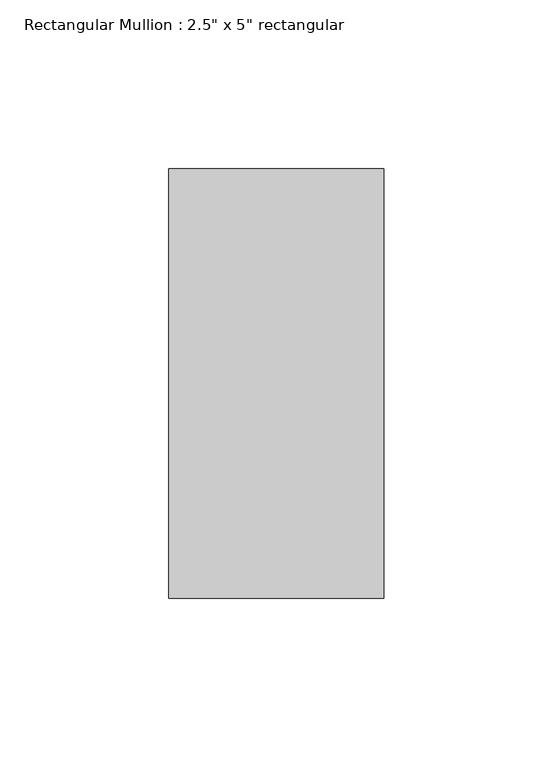
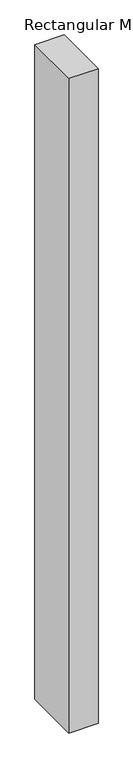
"""IFC4 building model written with IfcOpenShell, lengths in millimetres: member geometry."""

from ifc_helpers import new_model, si_unit, frame, origin, place, context, project, spatial, polyline, outline, extrude, source, transform, mapped, element, save


def member_0c2b78d7(model_context):
    return source(origin(), model_context, "Body", "SweptSolid", [
        extrude(outline(polyline([(0.0, 63.5), (0.0, -63.5), (-63.5, -63.5), (-63.5, 63.5), (0.0, 63.5)])), frame((0.0, 0.0, -1499.362181), z_axis=(0.0, 0.0, 1.0), x_axis=(1.0, 0.0, 0.0)), (0.0, 0.0, 1.0), 1499.362181),
    ])


if __name__ == "__main__":
    model = new_model("IFC4")
    model_context = context("Model", 3, world=origin())
    ifc_project = project(units=[si_unit("LENGTHUNIT", "METRE", prefix="MILLI")], contexts=[model_context])
    site = spatial("IfcSite", under=ifc_project)
    building = spatial("IfcBuilding", under=site)
    placement = place(None, origin())
    member_shape = member_0c2b78d7(model_context)
    element("IfcMember", 1, ObjectType="Rectangular Mullion : 2.5\" x 5\" rectangular", at=placement, inside=building, context=model_context, shape_type="MappedRepresentation", body=[
        mapped(member_shape, transform((0.0, 0.0, 0.0), x_axis=(1.0, 0.0, 0.0), y_axis=(0.0, 1.0, 0.0), z_axis=(0.0, 0.0, 1.0))),
    ])
    save(model, "model.ifc")

# Revit data of these elements
# Type "Rectangular Mullion : 2.5\" x 5\" rectangular"
#   built-in parameter 1007304 = 0.416667 (stored number, unit not read)
#   built-in parameter 1007301 = 0.104167 (stored number, unit not read)
#   built-in parameter 1007300 = 0.104167 (stored number, unit not read)
# Element 1 (IfcMember, "Rectangular Mullion : 2.5\" x 5\" rectangular")
#   Materials on its faces: "Aluminum"
# Materials
#   "Aluminum": class "Metal", colour RGB 247 247 247, transparency 0, Description = "Aluminum 6061", Cost = 0
